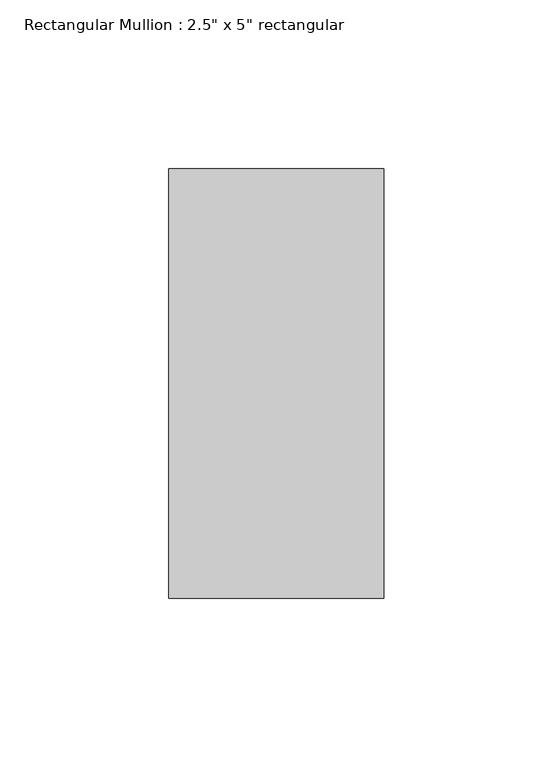
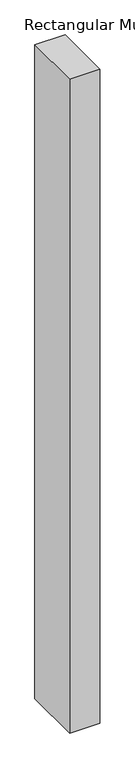
"""IFC4 building model written with IfcOpenShell, lengths in millimetres: member geometry."""

from ifc_helpers import new_model, si_unit, frame, origin, place, context, project, spatial, polyline, outline, extrude, source, transform, mapped, element, save


def member_ce41b455(model_context):
    return source(origin(), model_context, "Body", "SweptSolid", [
        extrude(outline(polyline([(0.0, 63.5), (0.0, -63.5), (-63.5, -63.5), (-63.5, 63.5), (0.0, 63.5)])), frame((0.0, 0.0, -1456.6512079), z_axis=(0.0, 0.0, 1.0), x_axis=(1.0, 0.0, 0.0)), (0.0, 0.0, 1.0), 1456.6512079),
    ])


if __name__ == "__main__":
    model = new_model("IFC4")
    model_context = context("Model", 3, world=origin())
    ifc_project = project(units=[si_unit("LENGTHUNIT", "METRE", prefix="MILLI")], contexts=[model_context])
    site = spatial("IfcSite", under=ifc_project)
    building = spatial("IfcBuilding", under=site)
    placement = place(None, origin())
    member_shape = member_ce41b455(model_context)
    element("IfcMember", 1, ObjectType="Rectangular Mullion : 2.5\" x 5\" rectangular", at=placement, inside=building, context=model_context, shape_type="MappedRepresentation", body=[
        mapped(member_shape, transform((0.0, 0.0, 0.0), x_axis=(1.0, 0.0, 0.0), y_axis=(0.0, 1.0, 0.0), z_axis=(0.0, 0.0, 1.0))),
    ])
    save(model, "model.ifc")

# Revit data of these elements
# Type "Rectangular Mullion : 2.5\" x 5\" rectangular"
#   built-in parameter 1007304 = 0.416667 (stored number, unit not read)
#   built-in parameter 1007301 = 0.104167 (stored number, unit not read)
#   built-in parameter 1007300 = 0.104167 (stored number, unit not read)
# Element 1 (IfcMember, "Rectangular Mullion : 2.5\" x 5\" rectangular")
#   Materials on its faces: "Aluminum"
# Materials
#   "Aluminum": class "Metal", colour RGB 247 247 247, transparency 0, Description = "Aluminum 6061", Cost = 0
